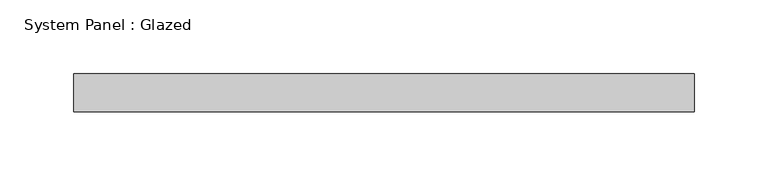
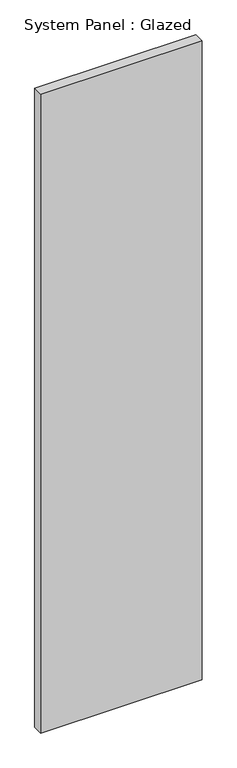
"""IFC4 building model written with IfcOpenShell, lengths in millimetres: plate geometry, System Panel : Glazed."""

from ifc_helpers import new_model, si_unit, origin, origin_with_axes, place, context, project, spatial, polyline, outline, extrude, source, transform, mapped, element, save


def system_panel_glazed_4b6a6dc2(model_context):
    return source(origin(), model_context, "Body", "SweptSolid", [
        extrude(outline(polyline([(209.55, 19.05), (-209.55, 19.05), (-209.55, 44.45), (209.55, 44.45), (209.55, 19.05)])), origin_with_axes(), (0.0, 0.0, 1.0), 1752.6),
    ])


if __name__ == "__main__":
    model = new_model("IFC4")
    model_context = context("Model", 3, world=origin())
    ifc_project = project(units=[si_unit("LENGTHUNIT", "METRE", prefix="MILLI")], contexts=[model_context])
    site = spatial("IfcSite", under=ifc_project)
    building = spatial("IfcBuilding", under=site)
    placement = place(None, origin())
    system_panel_glazed_shape = system_panel_glazed_4b6a6dc2(model_context)
    element("IfcPlate", 1, ObjectType="System Panel : Glazed", at=placement, inside=building, context=model_context, shape_type="MappedRepresentation", body=[
        mapped(system_panel_glazed_shape, transform((0.0, 0.0, 0.0), x_axis=(1.0, 0.0, 0.0), y_axis=(0.0, 1.0, 0.0), z_axis=(0.0, 0.0, 1.0))),
    ])
    save(model, "model.ifc")

# Revit data of these elements
# Type "System Panel : Glazed"
#   Construction Type Id = "GSP4R"
#   Analytic Construction = "1/8 in Pilkington single glazing"
#   Visual Light Transmittance = 0.9
#   Solar Heat Gain Coefficient = 0.86
#   Heat Transfer Coefficient (U) = 1.18115 BTU/(h·ft²·°F)
#   Define Thermal Properties by = 1
# Element 1 (IfcPlate, "System Panel : Glazed")
#   Materials on its faces: "Glass"
# Materials
#   "Glass": class "Glass", colour RGB 0 128 192, transparency 0.75, Description = "Soda Lime Glass", Cost = 0
